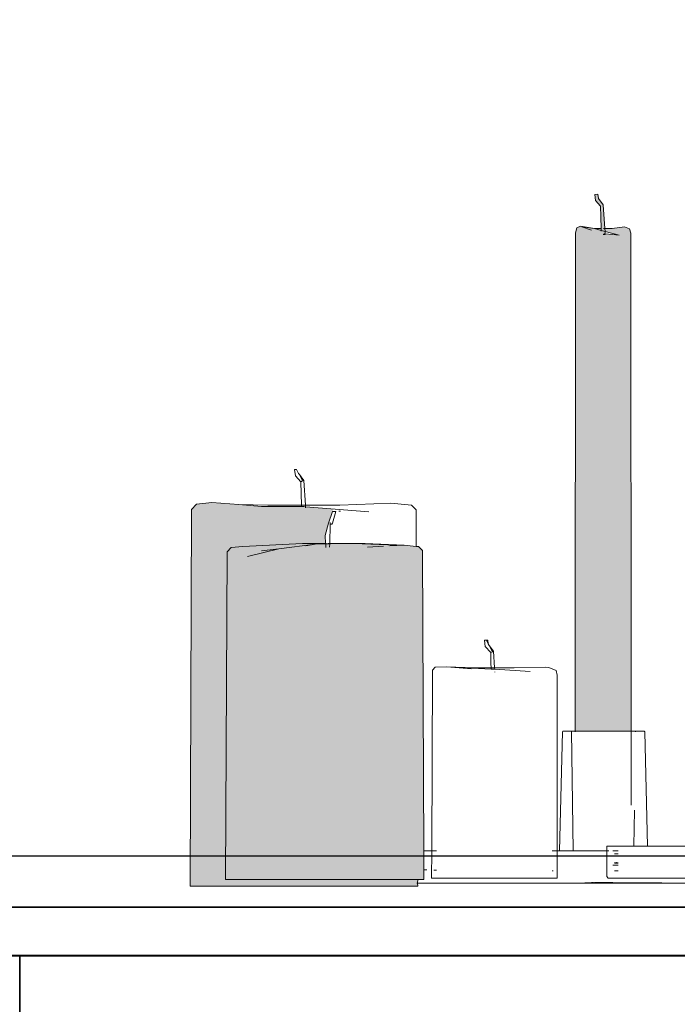
# Model space of a CAD drawing. Units: millimetres. Extents: x 446512 to 447461, y 70395 to 70610.
# Tile 14 of 39: x 446699.43 to 446706.19, y 70472.88 to 70483.01. Entities that reach past the tile are written whole.
import ezdxf

# ---------------------------------------------------------------- set-up
doc = ezdxf.new("R2010")
doc.units = ezdxf.units.MM
for name, color, linetype, lineweight in [('A-ANNO-DIMS', 2, 'Continuous', 18), ('A-FURN', 7, 'Continuous', 35), ('A-FURN-DECO', 8, 'Continuous', 13), ('A-FURN-PATT', 38, 'Continuous', 13)]:
    doc.layers.add(name, color=color, linetype=linetype, lineweight=lineweight)
doc.styles.get("Standard").update_dxf_attribs({"font": 'arial.ttf'})
doc.dimstyles.get("Standard").update_dxf_attribs({"dimtxt": 0.18, "dimasz": 0.18, "dimexe": 0.18, "dimexo": 0.0625, "dimgap": 0.09, "dimtad": 0, "dimtih": 1, "dimtoh": 1, "dimdec": 4, "dimzin": 0, "dimdsep": 46, "dimtxsty": 'Standard', "dimcen": 0.09, "dimadec": 0, "dimazin": 0, "dimtfac": 1, "dimtdec": 4, "dimtofl": 0, "dimtmove": 0, "dimatfit": 3, "dimfxl": 1, "dimtolj": 1, "dimtzin": 0, "dimarcsym": 0})

# ---------------------------------------------------------------- blocks, each defined once
blk = doc.blocks.new('*D32')
at = {"layer": 'A-ANNO-DIMS', "color": 0, "lineweight": -2, "transparency": 16777216}
for p, q in [((446730.76, 70474.405), (446678.043, 70474.405)), ((446678.223, 70474.225), (446678.223, 70474.075)), ((446678.223, 70473.562), (446678.223, 70473.711)), ((446728.946, 70473.382), (446678.043, 70473.382))]:
    blk.add_line(p, q, dxfattribs=at)
at = {"layer": 'A-ANNO-DIMS', "color": 0, "transparency": 16777216}
for points in [[(446678.193, 70474.225), (446678.253, 70474.225), (446678.223, 70474.405)], [(446678.193, 70473.562), (446678.253, 70473.562), (446678.223, 70473.382)]]:
    blk.add_solid(points, dxfattribs=at)
at = {"layer": 'Defpoints', "color": 0, "transparency": 16777216}
for p in [(446730.822, 70474.405), (446678.223, 70473.382), (446729.008, 70473.382)]:
    blk.add_point(p, dxfattribs=at)
at = {"layer": 'A-ANNO-DIMS', "color": 0, "transparency": 16777216, "insert": (446678.223, 70473.893), "char_height": 0.18, "attachment_point": 5}
blk.add_mtext('\\A1;1.02', dxfattribs=at)

msp = doc.modelspace()

# ---------------------------------------------------------------- hatches: boundary and pattern name
at = {"layer": 'A-FURN-PATT'}
h = msp.add_hatch(color=256, dxfattribs=at)
h.dxf.hatch_style = 1
h.paths.add_polyline_path([(446705.7043, 70475.6894), (446705.6867, 70475.6894), (446705.68, 70475.6894), (446705.652, 70475.6894), (446705.6322, 70475.6894), (446705.6158, 70475.6894), (446705.5769, 70475.6894), (446705.5386, 70475.6894), (446705.5161, 70475.6894), (446705.4574, 70475.6894), (446705.4521, 70475.6894), (446705.4197, 70475.6894), (446705.4162, 70475.6894), (446705.3557, 70475.6894), (446705.3348, 70475.6894), (446705.2947, 70475.6894), (446705.2427, 70475.6893), (446705.223, 70475.6894), (446705.2209, 70475.6894), (446705.2194, 70475.6894), (446705.2167, 70475.6894), (446705.2139, 70475.6894), (446705.1733, 70475.6894), (446705.1434, 70475.6893), (446705.1466, 70480.8149), (446705.1587, 70480.8664), (446705.1978, 70480.8847), (446705.3397, 70480.8584), (446705.4097, 70480.8583), (446705.4065, 70480.981), (446705.4042, 70481.0881), (446705.3508, 70481.1471), (446705.3429, 70481.2096), (446705.3746, 70481.2113), (446705.3819, 70481.1683), (446705.4319, 70481.1015), (446705.4482, 70480.8582), (446705.5217, 70480.8581), (446705.6504, 70480.8776), (446705.7027, 70480.8576), (446705.7147, 70480.8112), (446705.7183, 70475.6894), (446705.7299, 70475.6892), (446705.7467, 70475.6894), (446705.7183, 70475.6894), (446705.7183, 70475.6894), (446705.7135, 70475.6894)])
h.paths.add_polyline_path([(446705.4501, 70480.8298), (446705.5953, 70480.7922), (446705.4518, 70480.8042), (446705.4524, 70480.7961), (446705.4367, 70480.7969), (446705.4524, 70480.7965)], flags=16)
h.paths.add_polyline_path([(446702.6569, 70477.9751), (446702.3519, 70477.999), (446702.3274, 70477.999), (446701.9188, 70477.9993), (446701.6827, 70478.0201), (446701.4055, 70478.043), (446701.2463, 70478.024), (446701.1973, 70477.9703), (446701.1809, 70474.0948), (446703.5228, 70474.0948), (446703.522, 70474.1286), (446703.514, 70474.1286), (446703.522, 70474.1286), (446703.5225, 70474.1653), (446701.547, 70474.1653), (446701.5612, 70477.5357), (446701.6039, 70477.5792), (446701.7238, 70477.5898), (446702.3373, 70477.6192), (446702.5757, 70477.6192), (446702.571, 70477.7032), (446702.6044, 70477.829)])
h = msp.add_hatch(color=256, dxfattribs=at)
h.dxf.hatch_style = 1
h.paths.add_polyline_path([(446703.5722, 70477.5476), (446703.5295, 70477.5904), (446703.508, 70477.5904), (446703.383, 70477.6041), (446703.3062, 70477.6039), (446702.8621, 70477.6193), (446702.7177, 70477.6193), (446702.6174, 70477.6163), (446702.576, 70477.615), (446702.5757, 70477.6192), (446702.3373, 70477.6192), (446701.7238, 70477.5898), (446701.6039, 70477.5792), (446701.5612, 70477.5357), (446701.547, 70474.1653), (446703.5225, 70474.1653), (446703.5865, 70474.1653), (446703.5861, 70474.2632), (446703.5852, 70474.4594)])
h.paths.add_polyline_path([(446715.9764, 70475.5286), (446716.1565, 70476.0766), (446716.2492, 70476.4728), (446716.2873, 70476.8422), (446716.2666, 70477.0104), (446716.236, 70477.1061), (446716.1173, 70477.332), (446715.9979, 70477.4937), (446715.8249, 70477.6853), (446715.558, 70477.9316), (446715.2321, 70478.1882), (446714.7182, 70478.5467), (446714.5954, 70478.6535), (446714.3996, 70478.8999), (446714.3461, 70479.0185), (446714.3253, 70479.1028), (446714.3286, 70480.1095), (446714.368, 70480.1364), (446714.3744, 70480.152), (446714.3709, 70480.1808), (446714.3551, 70480.2131), (446714.3271, 70480.2359), (446714.3039, 70480.2478), (446714.2782, 70480.2478), (446714.259, 70480.2458), (446714.2432, 70480.2391), (446714.2375, 70480.2284), (446714.2369, 70480.2218), (446714.2301, 70480.2478), (446713.8255, 70480.2478), (446713.8277, 70480.2375), (446713.8104, 70480.2458), (446713.7912, 70480.2478), (446713.7655, 70480.2478), (446713.738, 70480.2359), (446713.7079, 70480.2028), (446713.6947, 70480.1567), (446713.6986, 70480.1448), (446713.717, 70480.1274), (446713.7341, 70480.1112), (446713.7407, 70480.1049), (446713.7473, 70479.1348), (446713.7233, 70479.0185), (446713.6698, 70478.8999), (446713.5684, 70478.7546), (446713.4739, 70478.6535), (446713.3511, 70478.5467), (446712.8373, 70478.1882), (446712.5114, 70477.9316), (446712.4629, 70477.8868), (446712.2445, 70477.6853), (446712.0714, 70477.4937), (446711.9521, 70477.332), (446711.866, 70477.1682), (446711.8333, 70477.1061), (446711.7899, 70476.9473), (446711.7821, 70476.8422), (446711.8202, 70476.4728), (446711.8563, 70476.3184), (446711.9128, 70476.0766), (446712.093, 70475.5286), (446712.2916, 70475.0627), (446712.4529, 70474.7607), (446712.5622, 70474.5947), (446712.6434, 70474.4935), (446712.7522, 70474.3925), (446712.8451, 70474.3334), (446713.0597, 70474.2483), (446713.2189, 70474.2124), (446713.4296, 70474.1861), (446713.8128, 70474.1834), (446713.5915, 70474.1683), (446714.5392, 70474.1683), (446714.4414, 70474.1779), (446714.1836, 70474.1834), (446714.6098, 70474.1861), (446714.8353, 70474.2124), (446714.9266, 70474.2312), (446715.0097, 70474.2483), (446715.2243, 70474.3334), (446715.3172, 70474.3925), (446715.3727, 70474.4388), (446715.5072, 70474.5947), (446715.6164, 70474.7607), (446715.7778, 70475.0627)])
h.paths.add_polyline_path([(446719.9646, 70475.8685), (446719.9469, 70476.8426), (446719.9277, 70476.9944), (446719.8688, 70477.2155), (446719.7757, 70477.4048), (446719.7115, 70477.4967), (446719.566, 70477.6531), (446719.2165, 70477.9493), (446719.1289, 70478.0481), (446719.1777, 70478.067), (446719.1866, 70478.0815), (446719.1867, 70478.209), (446719.1598, 70478.218), (446719.1369, 70478.2173), (446719.1374, 70478.2174), (446719.0341, 70478.2174), (446718.8666, 70478.218), (446718.6447, 70478.218), (446718.418, 70478.2174), (446718.1448, 70478.2174), (446717.8911, 70478.218), (446717.8873, 70478.218), (446717.6401, 70478.2174), (446717.4215, 70478.2174), (446717.2754, 70478.218), (446717.1987, 70478.218), (446717.2097, 70478.2113), (446717.1243, 70478.2174), (446717.1135, 70478.2124), (446717.1091, 70478.2029), (446717.1111, 70478.0815), (446717.1185, 70478.0683), (446717.1615, 70478.0517), (446717.1433, 70478.0167), (446717.0812, 70477.9493), (446716.7317, 70477.6531), (446716.5862, 70477.4967), (446716.47, 70477.311), (446716.3975, 70477.1183), (446716.37, 70476.9944), (446716.3508, 70476.8426), (446716.3331, 70475.8685), (446716.374, 70475.0624), (446716.4146, 70474.8322), (446716.4608, 70474.6687), (446716.5046, 70474.5619), (446716.5765, 70474.4449), (446716.6659, 70474.36), (446716.7457, 70474.3103), (446716.8351, 70474.2702), (446717.0729, 70474.2085), (446717.2886, 70474.1864), (446717.3803, 70474.1864), (446717.4428, 70474.1846), (446717.4556, 70474.1862), (446718.0146, 70474.1842), (446718.1072, 70474.1795), (446718.1371, 70474.1802), (446718.1473, 70474.1804), (446718.1566, 70474.1797), (446718.1569, 70474.1797), (446718.1592, 70474.1795), (446718.303, 70474.1842), (446719.0393, 70474.1865), (446719.2248, 70474.2085), (446719.365, 70474.2387), (446719.4626, 70474.2702), (446719.552, 70474.3103), (446719.6318, 70474.36), (446719.7212, 70474.4449), (446719.7931, 70474.5619), (446719.8369, 70474.6687), (446719.8831, 70474.8322), (446719.9155, 70475.0156), (446719.9237, 70475.0624)])
h.paths.add_polyline_path([(446718.18, 70474.3158), (446717.2692, 70474.3158), (446717.2092, 70474.3107), (446717.3763, 70474.3107)], flags=16)
h.paths.add_polyline_path([(446717.572, 70474.3384), (446717.5676, 70474.3381), (446717.5691, 70474.3381)], flags=16)
h.paths.add_polyline_path([(446722.3965, 70475.7383), (446722.4453, 70475.7383), (446722.4564, 70475.7383), (446722.4729, 70475.7383), (446722.4785, 70475.7384), (446722.4797, 70475.7383), (446722.4831, 70475.7383), (446722.4841, 70475.7384), (446722.5211, 70475.7384), (446722.4906, 70475.7381), (446722.4906, 70475.7384), (446722.4864, 70475.7383), (446722.4853, 70475.7383), (446722.4831, 70475.7383), (446722.4819, 70475.7383), (446722.4797, 70475.7383), (446722.4618, 70475.7383), (446722.4401, 70475.7383), (446722.4015, 70475.7383), (446722.3964, 70475.7341), (446722.3682, 70474.5084), (446722.5299, 70474.5084), (446723.2721, 70474.5084), (446723.2439, 70475.7341), (446723.2391, 70475.7383), (446723.2067, 70475.7383), (446723.1904, 70475.7383), (446723.1824, 70475.7383), (446723.1499, 70475.7382), (446723.1499, 70475.7384), (446723.1407, 70475.7384), (446723.1819, 70475.7384), (446723.1732, 70475.7384), (446723.1824, 70475.7383), (446723.1957, 70475.7383), (446723.1982, 70475.7383), (446723.2002, 70475.7383), (446723.2067, 70475.7383), (446723.2439, 70475.7383), (446723.2721, 70474.5084), (446724.6768, 70474.5084), (446724.7369, 70474.5652), (446724.8426, 70474.7369), (446724.9068, 70474.8938), (446724.9747, 70475.1338), (446725.0344, 70475.4718), (446725.0943, 70476.6554), (446725.0683, 70478.0856), (446725.0402, 70478.3085), (446724.9998, 70478.4903), (446724.9537, 70478.6331), (446724.8934, 70478.7733), (446724.817, 70478.911), (446724.7228, 70479.046), (446724.5091, 70479.2756), (446724.1522, 70479.5853), (446723.9922, 70479.7544), (446723.8721, 70479.9071), (446723.7862, 70480.0401), (446723.6778, 70480.2901), (446723.6684, 70480.351), (446723.714, 70480.381), (446723.7245, 70480.398), (446723.7213, 70480.4391), (446723.7096, 70480.4663), (446723.6751, 70480.5056), (446723.6405, 70480.5215), (446723.5985, 70480.5218), (446723.5958, 70480.5218), (446722.1196, 70480.5215), (446721.2867, 70480.5218), (446721.2939, 70480.516), (446721.2184, 70480.5218), (446721.1844, 70480.5072), (446721.155, 70480.479), (446721.1354, 70480.4391), (446721.1312, 70480.4035), (446721.1408, 70480.3826), (446721.1891, 70480.3558), (446721.179, 70480.2901), (446721.0706, 70480.0401), (446720.9847, 70479.9071), (446720.8645, 70479.7544), (446720.7046, 70479.5853), (446720.3925, 70479.3145), (446720.3476, 70479.2756), (446720.248, 70479.1783), (446720.134, 70479.046), (446720.0397, 70478.911), (446719.9634, 70478.7733), (446719.9031, 70478.6331), (446719.857, 70478.4903), (446719.8165, 70478.3085), (446719.7884, 70478.0856), (446719.7757, 70477.4048), (446719.8688, 70477.2155), (446719.9277, 70476.9944), (446719.9469, 70476.8426), (446719.9646, 70475.8685), (446719.9237, 70475.0624), (446719.9155, 70475.0156), (446719.9499, 70474.8938), (446720.064, 70474.6452), (446720.1198, 70474.5652), (446720.1819, 70474.4977), (446720.2884, 70474.4145), (446720.3682, 70474.3675), (446720.4995, 70474.3087), (446720.6428, 70474.2625), (446720.8486, 70474.2181), (446720.8834, 70474.214), (446720.8836, 70474.3337), (446720.8838, 70474.5084), (446722.3682, 70474.5084)])
h.paths.add_polyline_path([(446722.5299, 70477.9863), (446722.5458, 70478.1272), (446722.5844, 70478.1453), (446722.7245, 70478.1193), (446722.7937, 70478.1192), (446722.7905, 70478.2404), (446722.7882, 70478.3461), (446722.7354, 70478.4044), (446722.7276, 70478.4661), (446722.759, 70478.4678), (446722.7662, 70478.4254), (446722.8155, 70478.3594), (446722.8317, 70478.1191), (446722.9042, 70478.119), (446723.0314, 70478.1383), (446723.0829, 70478.1185), (446723.0949, 70478.0727), (446723.0974, 70475.7384), (446723.1135, 70475.7383), (446723.104, 70475.7384), (446723.1025, 70475.7384), (446723.0987, 70475.7384), (446723.0974, 70475.7383), (446723.0719, 70475.7383), (446723.018, 70475.7384), (446723.0095, 70475.7382), (446722.9885, 70475.7384), (446722.9576, 70475.7383), (446722.9328, 70475.7384), (446722.9244, 70475.7383), (446722.8841, 70475.7383), (446722.8055, 70475.7384), (446722.802, 70475.7383), (446722.7415, 70475.7384), (446722.7206, 70475.7383), (446722.7104, 70475.7384), (446722.6518, 70475.7384), (446722.6431, 70475.7383), (446722.6067, 70475.7383), (446722.5537, 70475.7384), (446722.5299, 70475.7383)], flags=16)
h.paths.add_polyline_path([(446722.7937, 70478.1192), (446722.8317, 70478.1191), (446722.8336, 70478.0906), (446722.8358, 70478.0578), (446722.7952, 70478.0599), (446722.7946, 70478.0859)], flags=0)
h.paths.add_polyline_path([(446723.5789, 70480.5193), (446723.5569, 70480.5185), (446723.5487, 70480.509)], flags=16)

# ---------------------------------------------------------------- linework, layer by layer
at = {"layer": 'A-FURN'}
for p, q in [((446686.5728, 70473.3815), (446746.5728, 70473.3815)), ((446699.4288, 70473.3815), (446699.4288, 70453.3815))]:
    msp.add_line(p, q, dxfattribs=at)
for points in [[(446686.5728, 70493.3815), (446729.0084, 70493.3815), (446729.0084, 70473.3815), (446686.5728, 70473.3815)], [(446687.0728, 70492.8815), (446728.5084, 70492.8815), (446728.5084, 70473.8815), (446687.0728, 70473.8815)], [(446699.4288, 70473.3815), (446746.5728, 70473.3815), (446746.5728, 70453.3815), (446699.4288, 70453.3815)]]:
    msp.add_lwpolyline(points, close=True, dxfattribs=at)
at = {"layer": 'A-FURN-DECO'}
for p, q in [((446705.3746, 70481.2113), (446705.3429, 70481.2096)), ((446705.3508, 70481.1471), (446705.3429, 70481.2096)), ((446705.4042, 70481.0881), (446705.3508, 70481.1471)), ((446705.3819, 70481.1683), (446705.3746, 70481.2113)), ((446705.4319, 70481.1015), (446705.3819, 70481.1683)), ((446705.4065, 70480.981), (446705.4042, 70481.0881)), ((446705.4319, 70481.1015), (446705.4482, 70480.8582)), ((446705.4097, 70480.8583), (446705.4065, 70480.981)), ((446705.1466, 70480.8149), (446705.1587, 70480.8664)), ((446705.1978, 70480.8847), (446705.1587, 70480.8664)), ((446705.3397, 70480.8584), (446705.1978, 70480.8847)), ((446705.3114, 70480.8434), (446705.2109, 70480.8749)), ((446705.2109, 70480.8749), (446705.3397, 70480.8584)), ((446705.3397, 70480.8584), (446705.4097, 70480.8583)), ((446705.4102, 70480.8401), (446705.3397, 70480.8584)), ((446705.4102, 70480.8401), (446705.4097, 70480.8583)), ((446705.4501, 70480.8298), (446705.4102, 70480.8401)), ((446705.4104, 70480.8334), (446705.4102, 70480.8401)), ((446705.4348, 70480.8583), (446705.446, 70480.8583)), ((446705.4482, 70480.8582), (446705.5217, 70480.8581)), ((446705.4482, 70480.8582), (446705.4501, 70480.8298)), ((446705.5217, 70480.8581), (446705.6504, 70480.8776)), ((446705.6504, 70480.8776), (446705.7027, 70480.8576)), ((446705.7027, 70480.8576), (446705.7147, 70480.8112)), ((446705.1434, 70475.6894), (446705.1466, 70480.8149)), ((446705.4367, 70480.7969), (446705.4307, 70480.7972)), ((446705.4364, 70480.8055), (446705.4518, 70480.8042)), ((446705.4367, 70480.7969), (446705.4524, 70480.7965)), ((446705.5953, 70480.7922), (446705.4501, 70480.8298)), ((446705.4501, 70480.8298), (446705.4514, 70480.8114)), ((446705.4518, 70480.8042), (446705.4524, 70480.7965)), ((446705.4518, 70480.8042), (446705.5953, 70480.7922)), ((446705.7183, 70475.6894), (446705.7147, 70480.8112)), ((446702.2571, 70478.3811), (446702.2776, 70478.3822)), ((446702.2571, 70478.3811), (446702.2655, 70478.3164)), ((446702.2655, 70478.3164), (446702.3212, 70478.2549)), ((446702.2979, 70478.3385), (446702.2776, 70478.3822)), ((446702.3054, 70478.3285), (446702.2979, 70478.3385)), ((446702.35, 70478.2689), (446702.3054, 70478.3285)), ((446702.3391, 70478.2635), (446702.3054, 70478.3285)), ((446702.3212, 70478.2549), (446702.3391, 70478.2635)), ((446702.3212, 70478.2549), (446702.327, 70478.0155)), ((446702.3391, 70478.2635), (446702.35, 70478.2689)), ((446702.367, 70478.0155), (446702.35, 70478.2689)), ((446701.1973, 70477.9703), (446701.2463, 70478.024)), ((446701.2463, 70478.024), (446701.4055, 70478.043)), ((446701.4055, 70478.043), (446701.6827, 70478.0201)), ((446701.6827, 70478.0201), (446701.9819, 70478.0156)), ((446701.6827, 70478.0201), (446701.9172, 70477.9994)), ((446701.9172, 70477.9994), (446701.9301, 70477.9993)), ((446701.9301, 70477.9993), (446702.3274, 70477.999)), ((446701.9819, 70478.0156), (446702.327, 70478.0155)), ((446702.327, 70478.0155), (446702.3274, 70477.999)), ((446702.3274, 70477.999), (446702.3519, 70477.999)), ((446702.3356, 70478.0155), (446702.367, 70478.0155)), ((446702.3519, 70477.999), (446702.3682, 70477.9977)), ((446702.367, 70478.0155), (446702.7218, 70478.0154)), ((446702.3682, 70477.9977), (446702.367, 70478.0155)), ((446702.3682, 70477.9977), (446703.0211, 70477.9467)), ((446702.369, 70477.9856), (446702.3682, 70477.9977)), ((446703.245, 70478.0356), (446702.7218, 70478.0154)), ((446703.245, 70478.0356), (446703.4574, 70478.0148)), ((446703.5064, 70477.9665), (446703.4574, 70478.0148)), ((446701.1809, 70474.0948), (446701.1973, 70477.9703)), ((446702.6044, 70477.829), (446702.6473, 70477.9483)), ((446702.6454, 70477.8289), (446702.6813, 70477.9477)), ((446702.6473, 70477.9483), (446702.6813, 70477.9477)), ((446702.7101, 70477.9534), (446702.7276, 70477.953)), ((446703.508, 70477.5904), (446703.5064, 70477.9665)), ((446702.571, 70477.7032), (446702.6044, 70477.829)), ((446702.6222, 70477.8204), (446702.6174, 70477.6193)), ((446702.6237, 70477.8344), (446702.6222, 70477.8204)), ((446702.6222, 70477.8204), (446702.6402, 70477.8204)), ((446702.6402, 70477.8204), (446702.6454, 70477.8289)), ((446702.5757, 70477.6192), (446702.571, 70477.7032)), ((446702.3373, 70477.6192), (446701.7238, 70477.5898)), ((446702.4684, 70477.6118), (446702.0937, 70477.5641)), ((446702.3373, 70477.6192), (446702.5757, 70477.6192)), ((446702.3736, 70477.5948), (446702.4684, 70477.6118)), ((446702.4684, 70477.6118), (446702.576, 70477.615)), ((446702.5757, 70477.6192), (446702.5796, 70477.6192)), ((446702.576, 70477.615), (446702.5757, 70477.6192)), ((446702.576, 70477.615), (446702.6174, 70477.6163)), ((446702.5781, 70477.5774), (446702.576, 70477.615)), ((446702.601, 70477.6192), (446702.6174, 70477.6193)), ((446702.6174, 70477.6163), (446702.6164, 70477.5822)), ((446702.6174, 70477.6193), (446702.7177, 70477.6193)), ((446702.6174, 70477.6163), (446702.7177, 70477.6193)), ((446702.6174, 70477.6193), (446702.6174, 70477.6163)), ((446702.7177, 70477.6193), (446702.7962, 70477.6216)), ((446702.7177, 70477.6193), (446702.8621, 70477.6193)), ((446702.7962, 70477.6216), (446702.8621, 70477.6193)), ((446702.8621, 70477.6193), (446702.9817, 70477.6194)), ((446702.8621, 70477.6193), (446703.3062, 70477.6039)), ((446702.9817, 70477.6194), (446703.383, 70477.6041)), ((446703.0057, 70477.582), (446703.17, 70477.5916)), ((446703.2368, 70477.5955), (446703.383, 70477.6041)), ((446703.383, 70477.6041), (446703.3062, 70477.6039)), ((446703.383, 70477.6041), (446703.508, 70477.5904)), ((446703.508, 70477.5904), (446703.5295, 70477.5904)), ((446703.5295, 70477.5904), (446703.5722, 70477.5476)), ((446701.547, 70474.1653), (446701.5612, 70477.5357)), ((446701.6039, 70477.5792), (446701.5612, 70477.5357)), ((446701.7238, 70477.5898), (446701.6039, 70477.5792)), ((446701.7709, 70477.4868), (446702.0937, 70477.5641)), ((446701.9144, 70477.5436), (446702.0937, 70477.5641)), ((446703.5722, 70477.5476), (446703.5852, 70474.4594)), ((446704.2302, 70476.6263), (446704.2095, 70476.6247)), ((446704.2178, 70476.5599), (446704.2095, 70476.6247)), ((446704.2302, 70476.6263), (446704.2427, 70476.6268)), ((446704.249, 70476.5897), (446704.2302, 70476.6263)), ((446704.249, 70476.5897), (446704.2427, 70476.6268)), ((446704.2503, 70476.5821), (446704.249, 70476.5897)), ((446704.2587, 70476.5708), (446704.249, 70476.5897)), ((446704.2587, 70476.5708), (446704.2503, 70476.5821)), ((446704.2178, 70476.5599), (446704.2736, 70476.4985)), ((446704.2915, 70476.507), (446704.2587, 70476.5708)), ((446704.3024, 70476.5125), (446704.2587, 70476.5708)), ((446704.2915, 70476.507), (446704.2736, 70476.4985)), ((446704.2762, 70476.3894), (446704.2736, 70476.4985)), ((446704.3024, 70476.5125), (446704.2915, 70476.507)), ((446704.3138, 70476.3428), (446704.3024, 70476.5125)), ((446704.2759, 70476.3869), (446704.2762, 70476.3894)), ((446704.2759, 70476.3869), (446704.2771, 70476.3428)), ((446703.6664, 70474.4594), (446703.6742, 70476.3179)), ((446703.6742, 70476.3179), (446703.7013, 70476.3475)), ((446703.8184, 70476.3523), (446703.7013, 70476.3475)), ((446704.0776, 70476.3315), (446703.8184, 70476.3523)), ((446704.1071, 70476.3429), (446703.8184, 70476.3523)), ((446703.8184, 70476.3523), (446704.2775, 70476.3282)), ((446704.2771, 70476.3428), (446704.1071, 70476.3429)), ((446704.2771, 70476.3428), (446704.2775, 70476.3282)), ((446704.3138, 70476.3428), (446704.2771, 70476.3428)), ((446704.2775, 70476.3282), (446704.3112, 70476.3272)), ((446704.3148, 70476.3269), (446704.3112, 70476.3272)), ((446704.3148, 70476.3269), (446704.3138, 70476.3428)), ((446704.5153, 70476.3427), (446704.3138, 70476.3428)), ((446704.6803, 70476.3048), (446704.3148, 70476.3269)), ((446704.3167, 70476.2983), (446704.3166, 70476.3)), ((446704.8333, 70476.3477), (446704.5153, 70476.3427)), ((446704.8729, 70476.3458), (446704.8333, 70476.3477)), ((446704.9481, 70476.3158), (446704.8729, 70476.3458)), ((446704.9571, 70476.2657), (446704.9481, 70476.3158)), ((446704.9571, 70476.2657), (446704.9571, 70474.4594)), ((446704.9824, 70474.4594), (446705.0106, 70475.6851)), ((446705.0106, 70475.6851), (446705.0154, 70475.6894)), ((446705.0404, 70475.6894), (446705.0154, 70475.6894)), ((446705.0478, 70475.6894), (446705.0404, 70475.6894)), ((446705.0543, 70475.6894), (446705.0478, 70475.6894)), ((446705.0564, 70475.6894), (446705.0543, 70475.6894)), ((446705.0588, 70475.6894), (446705.0564, 70475.6894)), ((446705.0735, 70475.6894), (446705.0588, 70475.6894)), ((446705.0735, 70475.6894), (446705.0878, 70475.6894)), ((446705.0878, 70475.6894), (446705.0955, 70475.6894)), ((446705.0955, 70475.6894), (446705.099, 70475.6894)), ((446705.099, 70475.6894), (446705.1046, 70475.6894)), ((446705.1046, 70475.6894), (446705.1227, 70474.4594)), ((446705.1046, 70475.6894), (446705.1138, 70475.6894)), ((446705.1221, 70475.6894), (446705.1138, 70475.6894)), ((446705.1241, 70475.6894), (446705.1221, 70475.6894)), ((446705.1434, 70475.6894), (446705.1241, 70475.6894)), ((446705.1434, 70475.6894), (446705.1521, 70475.6894)), ((446705.1434, 70475.6851), (446705.1434, 70475.6894)), ((446705.1521, 70475.6894), (446705.1546, 70475.6894)), ((446705.1546, 70475.6894), (446705.1661, 70475.6894)), ((446705.1661, 70475.6894), (446705.1702, 70475.6894)), ((446705.1702, 70475.6894), (446705.1733, 70475.6894)), ((446705.1733, 70475.6894), (446705.1888, 70475.6894)), ((446705.1987, 70475.6894), (446705.1888, 70475.6894)), ((446705.1987, 70475.6894), (446705.2139, 70475.6894)), ((446705.2167, 70475.6894), (446705.2139, 70475.6894)), ((446705.2194, 70475.6894), (446705.2167, 70475.6894)), ((446705.2209, 70475.6894), (446705.2194, 70475.6894)), ((446705.223, 70475.6894), (446705.2209, 70475.6894)), ((446705.2275, 70475.6894), (446705.223, 70475.6894)), ((446705.2275, 70475.6894), (446705.239, 70475.6894)), ((446705.2573, 70475.6894), (446705.239, 70475.6894)), ((446705.2573, 70475.6894), (446705.2947, 70475.6894)), ((446705.3348, 70475.6894), (446705.2947, 70475.6894)), ((446705.3348, 70475.6894), (446705.3557, 70475.6894)), ((446705.3557, 70475.6894), (446705.4162, 70475.6894)), ((446705.4162, 70475.6894), (446705.4197, 70475.6894)), ((446705.4197, 70475.6894), (446705.4521, 70475.6894)), ((446705.4574, 70475.6894), (446705.4521, 70475.6894)), ((446705.4574, 70475.6894), (446705.5161, 70475.6894)), ((446705.5386, 70475.6894), (446705.5161, 70475.6894)), ((446705.5386, 70475.6894), (446705.5769, 70475.6894)), ((446705.6158, 70475.6894), (446705.5769, 70475.6894)), ((446705.6158, 70475.6894), (446705.6322, 70475.6894)), ((446705.6322, 70475.6894), (446705.652, 70475.6894)), ((446705.652, 70475.6894), (446705.68, 70475.6894)), ((446705.68, 70475.6894), (446705.6867, 70475.6894)), ((446705.7043, 70475.6894), (446705.6867, 70475.6894)), ((446705.7043, 70475.6894), (446705.7135, 70475.6894)), ((446705.7135, 70475.6894), (446705.7183, 70475.6894)), ((446705.7185, 70474.9306), (446705.7183, 70475.6894)), ((446705.7207, 70475.6894), (446705.7183, 70475.6894)), ((446705.7294, 70475.6894), (446705.7207, 70475.6894)), ((446705.7308, 70475.6894), (446705.7294, 70475.6894)), ((446705.7321, 70475.6894), (446705.7308, 70475.6894)), ((446705.7321, 70475.6894), (446705.7334, 70475.6894)), ((446705.7378, 70475.6894), (446705.7334, 70475.6894)), ((446705.7391, 70475.6894), (446705.7378, 70475.6894)), ((446705.7413, 70475.6894), (446705.7391, 70475.6894)), ((446705.7434, 70475.6894), (446705.7413, 70475.6894)), ((446705.7467, 70475.6894), (446705.7434, 70475.6894)), ((446705.7502, 70475.6894), (446705.7467, 70475.6894)), ((446705.7517, 70475.6894), (446705.7502, 70475.6894)), ((446705.7517, 70475.6894), (446705.7549, 70475.6894)), ((446705.7529, 70475.6894), (446705.7517, 70475.6894)), ((446705.7549, 70475.6894), (446705.7529, 70475.6894)), ((446705.7549, 70475.6894), (446705.7573, 70475.6894)), ((446705.7606, 70475.6894), (446705.7573, 70475.6894)), ((446705.7641, 70475.6894), (446705.7606, 70475.6894)), ((446705.7641, 70475.6894), (446705.764, 70475.6851)), ((446705.7673, 70475.6894), (446705.7641, 70475.6894)), ((446705.7697, 70475.6894), (446705.7673, 70475.6894)), ((446705.7861, 70475.6894), (446705.7697, 70475.6894)), ((446705.792, 70475.6894), (446705.7861, 70475.6894)), ((446705.7953, 70475.6894), (446705.792, 70475.6894)), ((446705.7972, 70475.6894), (446705.7953, 70475.6894)), ((446705.7972, 70475.6894), (446705.8531, 70475.6894)), ((446705.8582, 70475.6851), (446705.8531, 70475.6894)), ((446705.8852, 70474.5084), (446705.8582, 70475.6851)), ((446705.7522, 70474.8782), (446705.7467, 70474.5084)), ((446703.5852, 70474.4594), (446703.5861, 70474.2632)), ((446703.5852, 70474.4594), (446703.6664, 70474.4594)), ((446703.6652, 70474.1799), (446703.6664, 70474.4594)), ((446703.6664, 70474.4594), (446703.7173, 70474.4594)), ((446704.905, 70474.4594), (446704.9571, 70474.4594)), ((446704.9571, 70474.4594), (446704.9571, 70474.1799)), ((446704.9571, 70474.4594), (446704.9824, 70474.4594)), ((446704.9824, 70474.4594), (446705.1227, 70474.4594)), ((446705.4675, 70474.4594), (446705.1227, 70474.4594)), ((446705.4671, 70474.1952), (446705.4675, 70474.4594)), ((446705.4675, 70474.4594), (446705.4675, 70474.5084)), ((446705.4675, 70474.5084), (446705.4845, 70474.5084)), ((446705.4675, 70474.4594), (446705.4895, 70474.4594)), ((446705.4872, 70474.5083), (446705.4845, 70474.5084)), ((446705.4872, 70474.5083), (446705.4896, 70474.5084)), ((446705.4896, 70474.5084), (446705.4899, 70474.5052)), ((446705.4896, 70474.5084), (446705.5283, 70474.5084)), ((446705.5851, 70474.4594), (446705.5282, 70474.4594)), ((446705.5283, 70474.5084), (446705.539, 70474.5083)), ((446705.539, 70474.5083), (446705.5473, 70474.5083)), ((446705.5473, 70474.5083), (446705.5735, 70474.5084)), ((446705.7467, 70474.5084), (446705.5735, 70474.5084)), ((446705.8852, 70474.5084), (446705.7467, 70474.5084)), ((446706.9074, 70474.5084), (446705.8852, 70474.5084)), ((446705.5471, 70474.4296), (446705.585, 70474.4296)), ((446703.5861, 70474.2632), (446703.6153, 70474.263)), ((446703.5861, 70474.2632), (446703.5865, 70474.1653)), ((446703.6897, 70474.2625), (446703.7166, 70474.2623)), ((446704.9058, 70474.2542), (446704.9173, 70474.2542)), ((446705.528, 70474.3123), (446705.5748, 70474.3123)), ((446705.5848, 70474.2541), (446705.5467, 70474.2541)), ((446705.5834, 70474.3324), (446705.5472, 70474.3324)), ((446705.5476, 70474.3384), (446705.5627, 70474.338)), ((446705.5477, 70474.3369), (446705.5627, 70474.338)), ((446705.5834, 70474.3324), (446705.5477, 70474.3336)), ((446705.5627, 70474.338), (446705.568, 70474.3384)), ((446705.568, 70474.3384), (446705.5849, 70474.3374)), ((446705.5748, 70474.3123), (446705.5849, 70474.3122)), ((446705.5849, 70474.3324), (446705.5834, 70474.3324)), ((446703.5225, 70474.1653), (446701.547, 70474.1653)), ((446703.522, 70474.1286), (446703.5225, 70474.1653)), ((446703.5865, 70474.1653), (446703.5225, 70474.1653)), ((446704.9571, 70474.1799), (446703.6652, 70474.1799)), ((446705.4819, 70474.1775), (446705.4671, 70474.1952)), ((446705.5986, 70474.1775), (446705.4819, 70474.1775)), ((446705.5986, 70474.1775), (446705.6709, 70474.1778)), ((446705.6724, 70474.1775), (446705.6709, 70474.1778)), ((446705.6724, 70474.1775), (446707.3711, 70474.1775)), ((446703.5228, 70474.0948), (446701.1809, 70474.0948)), ((446703.514, 70474.1286), (446703.522, 70474.1286)), ((446703.5292, 70474.1286), (446703.522, 70474.1286)), ((446703.5228, 70474.0948), (446703.522, 70474.1286)), ((446703.5292, 70474.1286), (446705.169, 70474.1286)), ((446705.3118, 70474.1325), (446705.169, 70474.1286)), ((446705.169, 70474.1286), (446705.357, 70474.1286)), ((446705.3324, 70474.1325), (446705.3118, 70474.1325)), ((446705.3404, 70474.1324), (446705.3324, 70474.1325)), ((446705.3437, 70474.1326), (446705.3404, 70474.1324)), ((446705.3508, 70474.1326), (446705.3437, 70474.1326)), ((446705.3571, 70474.1326), (446705.3508, 70474.1326)), ((446705.363, 70474.1326), (446705.357, 70474.1286)), ((446705.5117, 70474.1286), (446705.357, 70474.1286)), ((446705.363, 70474.1326), (446705.3571, 70474.1326)), ((446705.3662, 70474.1326), (446705.363, 70474.1326)), ((446705.371, 70474.1326), (446705.3662, 70474.1326)), ((446705.3838, 70474.1326), (446705.371, 70474.1326)), ((446705.3866, 70474.1327), (446705.3838, 70474.1326)), ((446705.3915, 70474.1326), (446705.3866, 70474.1327)), ((446705.3941, 70474.1327), (446705.3915, 70474.1326)), ((446705.3971, 70474.1326), (446705.3941, 70474.1327)), ((446705.3986, 70474.1328), (446705.3971, 70474.1326)), ((446705.4028, 70474.1328), (446705.3986, 70474.1328)), ((446705.4047, 70474.1327), (446705.4028, 70474.1328)), ((446705.4047, 70474.1327), (446705.4064, 70474.1328)), ((446705.4091, 70474.1328), (446705.4064, 70474.1328)), ((446705.4113, 70474.1327), (446705.4091, 70474.1328)), ((446705.4128, 70474.1327), (446705.4113, 70474.1327)), ((446705.4142, 70474.1327), (446705.4128, 70474.1327)), ((446705.4142, 70474.1327), (446705.4172, 70474.1328)), ((446705.4142, 70474.1327), (446705.4193, 70474.1327)), ((446705.4172, 70474.1328), (446705.4193, 70474.1327)), ((446705.4193, 70474.1327), (446705.4229, 70474.1327)), ((446705.4229, 70474.1327), (446705.4256, 70474.1328)), ((446705.4242, 70474.1328), (446705.4229, 70474.1327)), ((446705.427, 70474.1327), (446705.4242, 70474.1328)), ((446705.4256, 70474.1328), (446705.427, 70474.1327)), ((446705.427, 70474.1327), (446705.4306, 70474.1328)), ((446705.4306, 70474.1328), (446705.4327, 70474.1328)), ((446705.4327, 70474.1328), (446705.4344, 70474.1327)), ((446705.4368, 70474.1328), (446705.4344, 70474.1327)), ((446705.4382, 70474.1328), (446705.4368, 70474.1328)), ((446705.4368, 70474.1328), (446705.4399, 70474.1328)), ((446705.4411, 70474.1328), (446705.4382, 70474.1328)), ((446705.4399, 70474.1328), (446705.4411, 70474.1328)), ((446705.4411, 70474.1328), (446705.4443, 70474.1327)), ((446705.4443, 70474.1327), (446705.4458, 70474.1328)), ((446705.4484, 70474.1328), (446705.4458, 70474.1328)), ((446705.4458, 70474.1328), (446705.4472, 70474.1327)), ((446705.4472, 70474.1327), (446705.4484, 70474.1328)), ((446705.4508, 70474.1328), (446705.4484, 70474.1328)), ((446705.4508, 70474.1328), (446705.4543, 70474.1327)), ((446705.4543, 70474.1327), (446705.4579, 70474.1327)), ((446705.4579, 70474.1327), (446705.4596, 70474.1328)), ((446705.4596, 70474.1328), (446705.4623, 70474.1328)), ((446705.4647, 70474.1327), (446705.4623, 70474.1328)), ((446705.4647, 70474.1327), (446705.4661, 70474.1327)), ((446705.4661, 70474.1327), (446705.4675, 70474.1328)), ((446705.4675, 70474.1328), (446705.4702, 70474.1328)), ((446705.4702, 70474.1328), (446705.4738, 70474.1326)), ((446705.4738, 70474.1326), (446705.4764, 70474.1327)), ((446705.4909, 70474.1326), (446705.4764, 70474.1327)), ((446705.4909, 70474.1326), (446705.5117, 70474.1286)), ((446705.4909, 70474.1326), (446705.5103, 70474.1325)), ((446705.5103, 70474.1325), (446705.514, 70474.1326)), ((446705.5117, 70474.1286), (446705.8852, 70474.1286)), ((446705.514, 70474.1326), (446705.5252, 70474.1326)), ((446705.5252, 70474.1326), (446705.5293, 70474.1325)), ((446705.5293, 70474.1325), (446705.588, 70474.1324)), ((446705.588, 70474.1324), (446705.5927, 70474.1323)), ((446705.5927, 70474.1323), (446705.6043, 70474.1324)), ((446705.6043, 70474.1324), (446705.7796, 70474.1318)), ((446705.7796, 70474.1318), (446706.0351, 70474.1314)), ((446705.7796, 70474.1318), (446705.8852, 70474.1286)), ((446706.0663, 70474.1286), (446705.8852, 70474.1286)), ((446706.0351, 70474.1314), (446706.0663, 70474.1286)), ((446706.0663, 70474.1286), (446707.3564, 70474.1286))]:
    msp.add_line(p, q, dxfattribs=at)

# ---------------------------------------------------------------- dimensions: what is measured, and where the dimension line sits
at = {"layer": 'A-ANNO-DIMS'}
dim = msp.add_linear_dim(base=(446678.2228, 70473.3815), p1=(446730.8224, 70474.4047), p2=(446729.0084, 70473.3815), angle=90, dimstyle='Standard', override={"dimdec": 2, "dimlfac": 1, "dimrnd": 0, "dimzin": 0, "dimdsep": 46, "dimlunit": 2}, dxfattribs=at)
dim.commit()
dim.dimension.update_dxf_attribs({"geometry": '*D32', "text_midpoint": (446678.2228, 70473.8931)})

doc.saveas('drawing.dxf')
